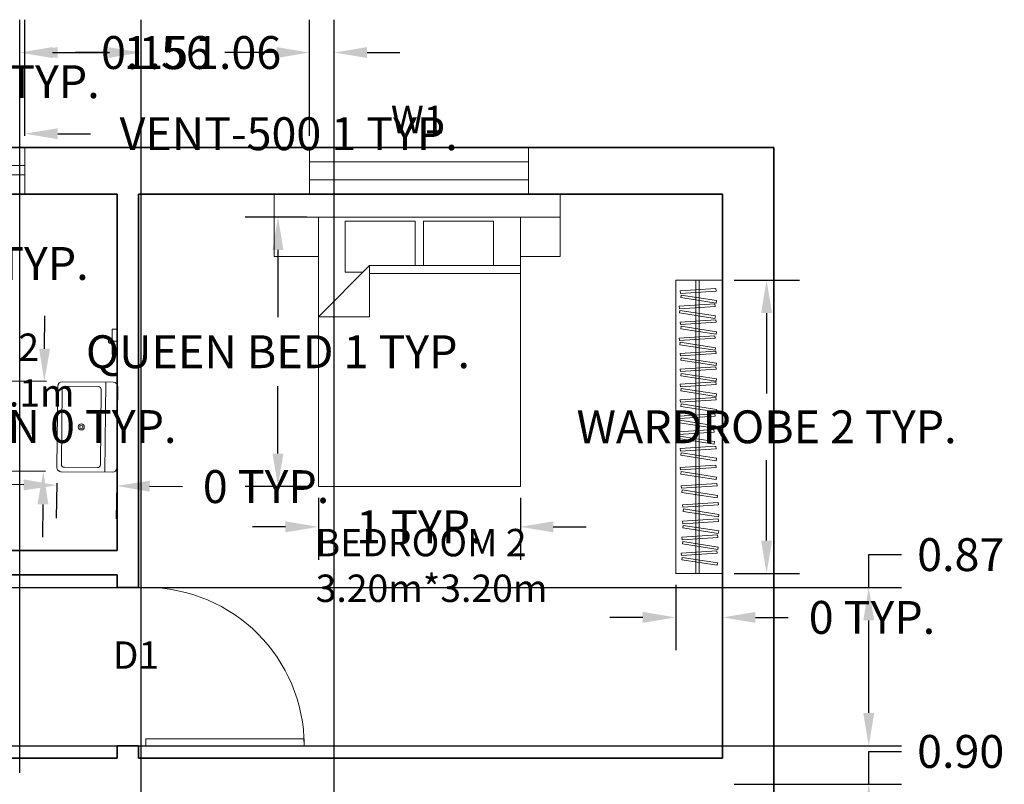
# Model space of a CAD drawing. Units: metres. Extents: x 1988.6 to 2001.1, y 2192 to 2202.5.
# Tile 6 of 6: x 1995.3 to 2000.6, y 2198.3 to 2202.5. Entities that reach past the tile are written whole.
import ezdxf

# ---------------------------------------------------------------- set-up
doc = ezdxf.new("R2010")
doc.units = ezdxf.units.M
for name, color, linetype, lineweight in [('A-ANNO-DIMS', 2, 'Continuous', 18), ('A-ANNO-TEXT', 7, 'Continuous', 18), ('A-AREA-IDEN', 7, 'Continuous', 18), ('A-DOOR', 3, 'Continuous', 18), ('A-FLOR-FIXT', 9, 'Continuous', 18), ('A-FURN', 9, 'Continuous', 15), ('A-GLAZ', 4, 'Continuous', 18), ('A-WALL', 7, 'Continuous', 35)]:
    doc.layers.add(name, color=color, linetype=linetype, lineweight=lineweight)
doc.styles.get("Standard").update_dxf_attribs({"font": 'arial.ttf'})
doc.dimstyles.get("Standard").update_dxf_attribs({"dimtxt": 0.18, "dimasz": 0.18, "dimexe": 0.18, "dimexo": 0.0625, "dimgap": 0.09, "dimtad": 0, "dimtih": 1, "dimtoh": 1, "dimdec": 4, "dimzin": 0, "dimdsep": 46, "dimtxsty": 'Standard', "dimcen": 0.09, "dimadec": 0, "dimazin": 0, "dimtfac": 1, "dimtdec": 4, "dimtofl": 0, "dimtmove": 0, "dimatfit": 3, "dimfxl": 1, "dimtolj": 1, "dimtzin": 0, "dimarcsym": 0})

# ---------------------------------------------------------------- blocks, each defined once
blk = doc.blocks.new('Bed - Queen')
for p, q in [((0, -80.00003), (0, 0)), ((0, 0), (59.99999, 0)), ((59.99999, 0), (59.99999, -80.00003)), ((7.99999, -1.2), (28.79998, -1.2)), ((7.99999, -14.4), (7.99999, -1.2)), ((28.79998, -1.2), (28.79998, -14.4)), ((31.19999, -1.2), (51.99999, -1.2)), ((31.19999, -14.4), (31.19999, -1.2)), ((51.99999, -1.2), (51.99999, -16.4)), ((0, -14.4), (44.8, -14.4)), ((59.99999, -29.6), (44.8, -14.4)), ((44.8, -14.4), (44.8, -29.6)), ((44.8, -16.8), (0, -16.8)), ((51.99999, -16.4), (46.79936, -16.4)), ((44.8, -29.6), (59.99999, -29.6)), ((59.99999, -80.00003), (0, -80.00003))]:
    blk.add_line(p, q)
blk = doc.blocks.new('Sink-single - 30 in top')
blk.add_line((-15, -3.999996), (15, -3.999996))
for points in [[(-13.5, 0), (13.5, 0)], [(-15, -18.499996), (-15, -1.5)], [(15, -1.5), (15, -18.499996)], [(-13.5, -17.499996), (-13.5, -6.499996)], [(-12.5, -5.499996), (12.5, -5.499996)], [(13.5, -6.499996), (13.5, -17.499996)], [(12.5, -18.499996), (-12.5, -18.499996)], [(13.5, -19.999996), (-13.5, -19.999996)]]:
    blk.add_lwpolyline(points)
for radius in [1, 0.5]:
    blk.add_circle((0, -11.999996), radius)
for centre, radius, start, end in [((-13.5, -1.5), 1.5, 90, 180), ((13.5, -1.5), 1.5, 0, 90), ((-12.5, -6.499996), 1, 90, 180), ((12.5, -6.499996), 1, 0, 90), ((-13.5, -18.499996), 1.5, 180, 270), ((-12.5, -17.499996), 1, 180, 270), ((12.5, -17.499996), 1, 270, 0), ((13.5, -18.499996), 1.5, 270, 0)]:
    blk.add_arc(centre, radius, start, end)
blk = doc.blocks.new('*U13')
for p, q in [((0, 0), (0, -6)), ((40, 0), (40, -6))]:
    blk.add_line(p, q)
blk.add_lwpolyline([(0, 0), (0, 40), (1.75, 40), (1.75, 0)], close=True)
blk.add_arc((0, 0), 40, 0, 90)
blk = doc.blocks.new('WIN-1200')
for p, q in [((-0.0002, 0.2568), (1.1998, 0.2568)), ((-0.0002, -0.0002), (-0.0002, 0.2568)), ((1.1998, 0.2568), (1.1998, -0.0002)), ((-0.0002, 0.1786), (1.1998, 0.1786)), ((-0.0002, 0.0793), (1.1998, 0.0793)), ((-0.0002, -0.0002), (1.1998, -0.0002))]:
    blk.add_line(p, q)
blk = doc.blocks.new('VENT-500')
for p, q in [((-0.0001, 0.2568), (-0.0001, -0.0002)), ((0.4999, 0.2568), (-0.0001, 0.2568)), ((0.4999, -0.0002), (0.4999, 0.2568)), ((0.4999, 0.1568), (-0.0001, 0.1568)), ((-0.0001, 0.1068), (0.4999, 0.1068)), ((-0.0001, -0.0002), (0.4999, -0.0002))]:
    blk.add_line(p, q)
blk = doc.blocks.new('HEADBOARD-WITH-SIDE-TABLES')
for p, q in [((-0.0002, 0.3408), (-0.0002, 0.2164)), ((1.5674, 0.2164), (1.5674, 0.3408)), ((-0.0002, 0.2164), (1.5674, 0.2164)), ((-0.0002, 0.2164), (-0.0002, 0.0002)), ((1.5674, 0.2164), (1.5674, 0.0002)), ((-0.0002, 0.0002), (0.2181, 0.0002)), ((1.5674, 0.0002), (1.3249, 0.0002))]:
    blk.add_line(p, q)
blk = doc.blocks.new('WARDROBE-HANGING')
for p, q in [((0.0001, 1.6061), (0.2571, 1.6061)), ((0.0001, 1.6061), (0.0001, 0.0002)), ((0.1103, 1.6061), (0.1103, 0.0002)), ((0.1286, 1.6061), (0.1286, 0.0002)), ((0.2571, 1.6061), (0.2571, 0.0002)), ((0.2571, 0.0002), (0.0001, 0.0002))]:
    blk.add_line(p, q)
for points in [[(0.0252, 1.5475), (0.2208, 1.5602), (0.2217, 1.5468), (0.0261, 1.5341)], [(0.0296, 1.5242), (0.2233, 1.4943), (0.2212, 1.481), (0.0275, 1.5109)], [(0.0193, 1.4638), (0.2148, 1.4765), (0.2157, 1.4631), (0.0201, 1.4504)], [(0.0236, 1.4404), (0.2173, 1.4105), (0.2153, 1.3972), (0.0216, 1.4272)], [(0.0252, 1.377), (0.2208, 1.3897), (0.2217, 1.3763), (0.0261, 1.3636)], [(0.0296, 1.3537), (0.2233, 1.3238), (0.2212, 1.3105), (0.0275, 1.3404)], [(0.0196, 1.2897), (0.2152, 1.3024), (0.2161, 1.289), (0.0205, 1.2763)], [(0.024, 1.2664), (0.2177, 1.2365), (0.2157, 1.2232), (0.022, 1.2531)], [(0.0252, 1.205), (0.2208, 1.2177), (0.2217, 1.2043), (0.0261, 1.1916)], [(0.0296, 1.1817), (0.2233, 1.1517), (0.2212, 1.1385), (0.0275, 1.1684)], [(0.0252, 1.1192), (0.2208, 1.1319), (0.2217, 1.1185), (0.0261, 1.1058)], [(0.0296, 1.0959), (0.2233, 1.066), (0.2212, 1.0527), (0.0275, 1.0827)], [(0.0252, 1.0365), (0.2208, 1.0492), (0.2217, 1.0358), (0.0261, 1.0231)], [(0.0296, 1.0132), (0.2233, 0.9833), (0.2212, 0.97), (0.0275, 0.9999)], [(0.0252, 0.9518), (0.2208, 0.9645), (0.2217, 0.9511), (0.0261, 0.9384)], [(0.0296, 0.9285), (0.2233, 0.8986), (0.2212, 0.8853), (0.0275, 0.9152)], [(0.0193, 0.8621), (0.2148, 0.8748), (0.2157, 0.8614), (0.0201, 0.8487)], [(0.0236, 0.8388), (0.2173, 0.8089), (0.2153, 0.7956), (0.0216, 0.8255)], [(0.0141, 0.7752), (0.2097, 0.7879), (0.2106, 0.7745), (0.015, 0.7618)], [(0.0185, 0.7519), (0.2122, 0.722), (0.2101, 0.7087), (0.0164, 0.7386)], [(0.0252, 0.6841), (0.2208, 0.6968), (0.2217, 0.6834), (0.0261, 0.6707)], [(0.0296, 0.6608), (0.2233, 0.6309), (0.2212, 0.6176), (0.0275, 0.6475)], [(0.0252, 0.5812), (0.2208, 0.5939), (0.2217, 0.5805), (0.0261, 0.5678)], [(0.0296, 0.5578), (0.2233, 0.5279), (0.2212, 0.5146), (0.0275, 0.5446)], [(0.0307, 0.4806), (0.2263, 0.4933), (0.2272, 0.4799), (0.0316, 0.4672)], [(0.0351, 0.4573), (0.2288, 0.4273), (0.2268, 0.4141), (0.0331, 0.444)], [(0.0379, 0.3765), (0.2335, 0.3892), (0.2344, 0.3758), (0.0388, 0.3631)], [(0.0423, 0.3532), (0.236, 0.3232), (0.2339, 0.31), (0.0403, 0.3399)], [(0.0375, 0.286), (0.2331, 0.2987), (0.234, 0.2853), (0.0384, 0.2726)], [(0.0419, 0.2627), (0.2356, 0.2327), (0.2335, 0.2195), (0.0399, 0.2494)], [(0.0342, 0.1981), (0.2298, 0.2108), (0.2307, 0.1974), (0.0351, 0.1847)], [(0.0386, 0.1748), (0.2323, 0.1448), (0.2303, 0.1316), (0.0366, 0.1615)], [(0.0307, 0.1115), (0.2263, 0.1242), (0.2272, 0.1108), (0.0316, 0.0981)], [(0.0351, 0.0882), (0.2288, 0.0583), (0.2268, 0.045), (0.0331, 0.0749)]]:
    blk.add_lwpolyline(points, close=True)
blk = doc.blocks.new('BATH-WALL-FITTING')
for p, q in [((-0.0001, 0.0002), (-0.0001, 0.138)), ((-0.0001, 0.138), (0.028, 0.138)), ((0.028, 0.1375), (0.028, 0.0002)), ((-0.0001, 0.0715), (0.028, 0.0715)), ((0.028, 0.0002), (-0.0001, 0.0002))]:
    blk.add_line(p, q)
blk.add_circle((0.0382, 0.0715), 0.0103)
blk = doc.blocks.new('*D24')
at = {"layer": 'A-ANNO-DIMS', "color": 0, "lineweight": -2, "transparency": 16777216}
for p, q in [((1996.824, 2201.3724), (1996.4852, 2201.3724)), ((1996.6652, 2201.1924), (1996.6652, 2200.8231)), ((1996.6652, 2200.0767), (1996.6652, 2200.4459)), ((1996.824, 2199.8967), (1996.4852, 2199.8967))]:
    blk.add_line(p, q, dxfattribs=at)
at = {"layer": 'A-ANNO-DIMS', "color": 0, "transparency": 16777216}
for points in [[(1996.6352, 2201.1924), (1996.6952, 2201.1924), (1996.6652, 2201.3724)], [(1996.6352, 2200.0767), (1996.6952, 2200.0767), (1996.6652, 2199.8967)]]:
    blk.add_solid(points, dxfattribs=at)
at = {"layer": 'Defpoints', "color": 0, "transparency": 16777216}
for p in [(1996.6652, 2201.3724), (1996.8865, 2201.3724), (1996.8865, 2199.8967)]:
    blk.add_point(p, dxfattribs=at)
at = {"layer": 'A-ANNO-DIMS', "color": 0, "transparency": 16777216, "insert": (1996.6652, 2200.6345), "char_height": 0.18, "attachment_point": 5}
blk.add_mtext('\\A1;QUEEN BED 1 TYP.', dxfattribs=at)
blk = doc.blocks.new('*D25')
at = {"layer": 'A-ANNO-DIMS', "color": 0, "lineweight": -2, "transparency": 16777216}
for p, q in [((1996.8865, 2199.8342), (1996.8865, 2199.4954)), ((1997.9932, 2199.8342), (1997.9932, 2199.4954)), ((1996.7065, 2199.6754), (1996.5265, 2199.6754)), ((1998.1732, 2199.6754), (1998.3532, 2199.6754))]:
    blk.add_line(p, q, dxfattribs=at)
at = {"layer": 'A-ANNO-DIMS', "color": 0, "transparency": 16777216}
for points in [[(1996.7065, 2199.7054), (1996.7065, 2199.6454), (1996.8865, 2199.6754)], [(1998.1732, 2199.7054), (1998.1732, 2199.6454), (1997.9932, 2199.6754)]]:
    blk.add_solid(points, dxfattribs=at)
at = {"layer": 'Defpoints', "color": 0, "transparency": 16777216}
for p in [(1996.8865, 2199.8967), (1997.9932, 2199.8967), (1996.8865, 2199.6754)]:
    blk.add_point(p, dxfattribs=at)
at = {"layer": 'A-ANNO-DIMS', "color": 0, "transparency": 16777216, "insert": (1997.4399, 2199.6754), "char_height": 0.18, "attachment_point": 5}
blk.add_mtext('\\A1;1 TYP.', dxfattribs=at)
blk = doc.blocks.new('*D28')
at = {"layer": 'A-ANNO-DIMS', "color": 0, "lineweight": -2, "transparency": 16777216}
for p, q in [((1995.3871, 2200.6513), (1995.3891, 2200.8313)), ((1995.3967, 2200.4712), (1995.2052, 2200.4733)), ((1995.3914, 2199.9779), (1995.1999, 2199.98)), ((1995.3779, 2199.7981), (1995.376, 2199.6181))]:
    blk.add_line(p, q, dxfattribs=at)
at = {"layer": 'A-ANNO-DIMS', "color": 0, "transparency": 16777216}
for points in [[(1995.3571, 2200.6517), (1995.4171, 2200.651), (1995.3852, 2200.4714)], [(1995.3479, 2199.7984), (1995.4079, 2199.7978), (1995.3799, 2199.9781)]]:
    blk.add_solid(points, dxfattribs=at)
at = {"layer": 'Defpoints', "color": 0, "transparency": 16777216}
for p in [(1995.4592, 2200.4706), (1995.3799, 2199.9781), (1995.4538, 2199.9773)]:
    blk.add_point(p, dxfattribs=at)
at = {"layer": 'A-ANNO-DIMS', "color": 0, "transparency": 16777216, "insert": (1995.3825, 2200.2247), "char_height": 0.18, "attachment_point": 5}
blk.add_mtext('\\A1;BASIN 0 TYP.', dxfattribs=at)
blk = doc.blocks.new('*D29')
at = {"layer": 'A-ANNO-DIMS', "color": 0, "lineweight": -2, "transparency": 16777216}
for p, q in [((1995.2731, 2199.9052), (1995.0931, 2199.9072)), ((1995.4532, 2199.9148), (1995.4511, 2199.7233)), ((1995.782, 2199.9112), (1995.78, 2199.7197)), ((1995.9619, 2199.8978), (1996.1419, 2199.8958))]:
    blk.add_line(p, q, dxfattribs=at)
at = {"layer": 'A-ANNO-DIMS', "color": 0, "transparency": 16777216}
for points in [[(1995.2734, 2199.9352), (1995.2727, 2199.8752), (1995.453, 2199.9033)], [(1995.9622, 2199.9278), (1995.9616, 2199.8678), (1995.7819, 2199.8997)]]:
    blk.add_solid(points, dxfattribs=at)
at = {"layer": 'Defpoints', "color": 0, "transparency": 16777216}
for p in [(1995.4538, 2199.9773), (1995.7827, 2199.9737), (1995.7819, 2199.8997)]:
    blk.add_point(p, dxfattribs=at)
at = {"layer": 'A-ANNO-DIMS', "color": 0, "transparency": 16777216, "insert": (1996.6, 2199.8958), "char_height": 0.18, "attachment_point": 5}
blk.add_mtext('\\A1;0 TYP.', dxfattribs=at)
blk = doc.blocks.new('*D34')
at = {"layer": 'A-ANNO-DIMS', "color": 0, "lineweight": -2, "transparency": 16777216}
for p, q in [((1994.7792, 2201.8163), (1994.7792, 2202.0088)), ((1995.2792, 2201.8163), (1995.2792, 2202.0088)), ((1994.5992, 2201.8288), (1994.4192, 2201.8288)), ((1995.4592, 2201.8288), (1995.6392, 2201.8288))]:
    blk.add_line(p, q, dxfattribs=at)
at = {"layer": 'A-ANNO-DIMS', "color": 0, "transparency": 16777216}
for points in [[(1994.5992, 2201.8588), (1994.5992, 2201.7988), (1994.7792, 2201.8288)], [(1995.4592, 2201.8588), (1995.4592, 2201.7988), (1995.2792, 2201.8288)]]:
    blk.add_solid(points, dxfattribs=at)
at = {"layer": 'Defpoints', "color": 0, "transparency": 16777216}
for p in [(1995.2792, 2201.8288), (1994.7792, 2201.7538), (1995.2792, 2201.7538)]:
    blk.add_point(p, dxfattribs=at)
at = {"layer": 'A-ANNO-DIMS', "color": 0, "transparency": 16777216, "insert": (1996.724, 2201.8288), "char_height": 0.18, "attachment_point": 5}
blk.add_mtext('\\A1;VENT-500 1 TYP.', dxfattribs=at)
blk = doc.blocks.new('*D35')
at = {"layer": 'A-ANNO-DIMS', "color": 0, "lineweight": -2, "transparency": 16777216}
for p, q in [((1994.7042, 2201.9338), (1994.7042, 2202.1138)), ((1994.7042, 2202.1138), (1994.8842, 2202.1138)), ((1994.7167, 2201.7538), (1994.5242, 2201.7538)), ((1994.7167, 2201.4968), (1994.5242, 2201.4968)), ((1994.7042, 2201.3168), (1994.7042, 2201.1368))]:
    blk.add_line(p, q, dxfattribs=at)
at = {"layer": 'A-ANNO-DIMS', "color": 0, "transparency": 16777216}
for points in [[(1994.6742, 2201.9338), (1994.7342, 2201.9338), (1994.7042, 2201.7538)], [(1994.6742, 2201.3168), (1994.7342, 2201.3168), (1994.7042, 2201.4968)]]:
    blk.add_solid(points, dxfattribs=at)
at = {"layer": 'Defpoints', "color": 0, "transparency": 16777216}
for p in [(1994.7042, 2201.7538), (1994.7792, 2201.7538), (1994.7792, 2201.4968)]:
    blk.add_point(p, dxfattribs=at)
at = {"layer": 'A-ANNO-DIMS', "color": 0, "transparency": 16777216, "insert": (1995.3424, 2202.1138), "char_height": 0.18, "attachment_point": 5}
blk.add_mtext('\\A1;0 TYP.', dxfattribs=at)
blk = doc.blocks.new('*D38')
at = {"layer": 'A-ANNO-DIMS', "color": 0, "lineweight": -2, "transparency": 16777216}
for p, q in [((1999.1632, 2201.0261), (1999.5216, 2201.0261)), ((1999.3416, 2200.8461), (1999.3416, 2200.4063)), ((1999.3416, 2199.6002), (1999.3416, 2200.04)), ((1999.1632, 2199.4202), (1999.5216, 2199.4202))]:
    blk.add_line(p, q, dxfattribs=at)
at = {"layer": 'A-ANNO-DIMS', "color": 0, "transparency": 16777216}
for points in [[(1999.3116, 2200.8461), (1999.3716, 2200.8461), (1999.3416, 2201.0261)], [(1999.3116, 2199.6002), (1999.3716, 2199.6002), (1999.3416, 2199.4202)]]:
    blk.add_solid(points, dxfattribs=at)
at = {"layer": 'Defpoints', "color": 0, "transparency": 16777216}
for p in [(1999.1007, 2201.0261), (1999.3416, 2201.0261), (1999.1007, 2199.4202)]:
    blk.add_point(p, dxfattribs=at)
at = {"layer": 'A-ANNO-DIMS', "color": 0, "transparency": 16777216, "insert": (1999.3416, 2200.2232), "char_height": 0.18, "attachment_point": 5}
blk.add_mtext('\\A1;WARDROBE 2 TYP.', dxfattribs=at)
blk = doc.blocks.new('*D39')
at = {"layer": 'A-ANNO-DIMS', "color": 0, "lineweight": -2, "transparency": 16777216}
for p, q in [((1998.8437, 2199.3577), (1998.8437, 2198.9993)), ((1999.1007, 2199.3577), (1999.1007, 2198.9993)), ((1998.6637, 2199.1793), (1998.4837, 2199.1793)), ((1999.2807, 2199.1793), (1999.4607, 2199.1793))]:
    blk.add_line(p, q, dxfattribs=at)
at = {"layer": 'A-ANNO-DIMS', "color": 0, "transparency": 16777216}
for points in [[(1998.6637, 2199.2093), (1998.6637, 2199.1493), (1998.8437, 2199.1793)], [(1999.2807, 2199.2093), (1999.2807, 2199.1493), (1999.1007, 2199.1793)]]:
    blk.add_solid(points, dxfattribs=at)
at = {"layer": 'Defpoints', "color": 0, "transparency": 16777216}
for p in [(1998.8437, 2199.4202), (1999.1007, 2199.4202), (1999.1007, 2199.1793)]:
    blk.add_point(p, dxfattribs=at)
at = {"layer": 'A-ANNO-DIMS', "color": 0, "transparency": 16777216, "insert": (1999.9188, 2199.1793), "char_height": 0.18, "attachment_point": 5}
blk.add_mtext('\\A1;0 TYP.', dxfattribs=at)
blk = doc.blocks.new('*D42')
at = {"layer": 'A-ANNO-DIMS', "color": 0, "lineweight": -2, "transparency": 16777216}
for p, q in [((1992.9081, 2200.938), (1992.9081, 2201.118)), ((1992.9081, 2201.118), (1993.0881, 2201.118)), ((1992.95, 2200.758), (1993.0881, 2200.758)), ((1992.95, 2200.6202), (1993.0881, 2200.6202)), ((1992.9081, 2200.4402), (1992.9081, 2200.2602))]:
    blk.add_line(p, q, dxfattribs=at)
at = {"layer": 'A-ANNO-DIMS', "color": 0, "transparency": 16777216}
for points in [[(1992.8781, 2200.938), (1992.9381, 2200.938), (1992.9081, 2200.758)], [(1992.8781, 2200.4402), (1992.9381, 2200.4402), (1992.9081, 2200.6202)]]:
    blk.add_solid(points, dxfattribs=at)
at = {"layer": 'Defpoints', "color": 0, "transparency": 16777216}
for p in [(1992.8875, 2200.758), (1992.9081, 2200.758), (1992.8875, 2200.6202)]:
    blk.add_point(p, dxfattribs=at)
at = {"layer": 'A-ANNO-DIMS', "color": 0, "transparency": 16777216, "insert": (1994.4511, 2201.118), "char_height": 0.18, "attachment_point": 5}
blk.add_mtext('\\A1;WALL FITTING 0 TYP.', dxfattribs=at)
blk = doc.blocks.new('*D57')
at = {"layer": 'A-ANNO-DIMS', "color": 0, "lineweight": -2, "transparency": 16777216}
for p, q in [((1995.2792, 2201.8163), (1995.2792, 2202.4533)), ((1996.8377, 2201.8163), (1996.8377, 2202.4533)), ((1995.4592, 2202.2733), (1995.7433, 2202.2733)), ((1996.6577, 2202.2733), (1996.3737, 2202.2733))]:
    blk.add_line(p, q, dxfattribs=at)
at = {"layer": 'A-ANNO-DIMS', "color": 0, "transparency": 16777216}
for points in [[(1995.4592, 2202.3033), (1995.4592, 2202.2433), (1995.2792, 2202.2733)], [(1996.6577, 2202.3033), (1996.6577, 2202.2433), (1996.8377, 2202.2733)]]:
    blk.add_solid(points, dxfattribs=at)
at = {"layer": 'Defpoints', "color": 0, "transparency": 16777216}
for p in [(1996.8377, 2202.2733), (1995.2792, 2201.7538), (1996.8377, 2201.7538)]:
    blk.add_point(p, dxfattribs=at)
at = {"layer": 'A-ANNO-DIMS', "color": 0, "transparency": 16777216, "insert": (1996.0585, 2202.2733), "char_height": 0.18, "attachment_point": 5}
blk.add_mtext('\\A1;1.56', dxfattribs=at)
blk = doc.blocks.new('*D71')
at = {"layer": 'A-ANNO-DIMS', "color": 0, "lineweight": -2, "transparency": 16777216}
for p, q in [((1999.9013, 2198.2651), (1999.9013, 2198.4451)), ((1999.9013, 2198.4451), (2000.0813, 2198.4451)), ((1999.1632, 2198.2651), (2000.0813, 2198.2651)), ((1999.9013, 2197.5493), (1999.9013, 2198.0851)), ((1999.4443, 2197.3693), (2000.0813, 2197.3693))]:
    blk.add_line(p, q, dxfattribs=at)
at = {"layer": 'A-ANNO-DIMS', "color": 0, "transparency": 16777216}
for points in [[(1999.8713, 2198.0851), (1999.9313, 2198.0851), (1999.9013, 2198.2651)], [(1999.8713, 2197.5493), (1999.9313, 2197.5493), (1999.9013, 2197.3693)]]:
    blk.add_solid(points, dxfattribs=at)
at = {"layer": 'Defpoints', "color": 0, "transparency": 16777216}
for p in [(1999.1007, 2198.2651), (1999.9013, 2198.2651), (1999.3818, 2197.3693)]:
    blk.add_point(p, dxfattribs=at)
at = {"layer": 'A-ANNO-DIMS', "color": 0, "transparency": 16777216, "insert": (2000.4048, 2198.4451), "char_height": 0.18, "attachment_point": 5}
blk.add_mtext('\\A1;0.90', dxfattribs=at)
blk = doc.blocks.new('*D72')
at = {"layer": 'A-ANNO-DIMS', "color": 0, "lineweight": -2, "transparency": 16777216}
for p, q in [((1999.9013, 2199.3431), (1999.9013, 2199.5231)), ((1999.9013, 2199.5231), (2000.0813, 2199.5231)), ((1992.7483, 2199.3431), (2000.0813, 2199.3431)), ((1999.9013, 2198.656), (1999.9013, 2199.1631)), ((1992.7483, 2198.476), (2000.0813, 2198.476))]:
    blk.add_line(p, q, dxfattribs=at)
at = {"layer": 'A-ANNO-DIMS', "color": 0, "transparency": 16777216}
for points in [[(1999.8713, 2199.1631), (1999.9313, 2199.1631), (1999.9013, 2199.3431)], [(1999.8713, 2198.656), (1999.9313, 2198.656), (1999.9013, 2198.476)]]:
    blk.add_solid(points, dxfattribs=at)
at = {"layer": 'Defpoints', "color": 0, "transparency": 16777216}
for p in [(1992.6858, 2199.3431), (1999.9013, 2199.3431), (1992.6858, 2198.476)]:
    blk.add_point(p, dxfattribs=at)
at = {"layer": 'A-ANNO-DIMS', "color": 0, "transparency": 16777216, "insert": (2000.4051, 2199.5231), "char_height": 0.18, "attachment_point": 5}
blk.add_mtext('\\A1;0.87', dxfattribs=at)
blk = doc.blocks.new('*D74')
at = {"layer": 'A-ANNO-DIMS', "color": 0, "lineweight": -2, "transparency": 16777216}
for p, q in [((1995.9155, 2195.9076), (1995.9155, 2202.4533)), ((1996.9733, 2195.9076), (1996.9733, 2202.4533)), ((1995.7355, 2202.2733), (1995.5555, 2202.2733)), ((1997.1533, 2202.2733), (1997.3333, 2202.2733))]:
    blk.add_line(p, q, dxfattribs=at)
at = {"layer": 'A-ANNO-DIMS', "color": 0, "transparency": 16777216}
for points in [[(1995.7355, 2202.3033), (1995.7355, 2202.2433), (1995.9155, 2202.2733)], [(1997.1533, 2202.3033), (1997.1533, 2202.2433), (1996.9733, 2202.2733)]]:
    blk.add_solid(points, dxfattribs=at)
at = {"layer": 'Defpoints', "color": 0, "transparency": 16777216}
for p in [(1996.9733, 2202.2733), (1995.9155, 2195.8451), (1996.9733, 2195.8451)]:
    blk.add_point(p, dxfattribs=at)
at = {"layer": 'A-ANNO-DIMS', "color": 0, "transparency": 16777216, "insert": (1996.4444, 2202.2733), "char_height": 0.18, "attachment_point": 5}
blk.add_mtext('\\A1;1.06', dxfattribs=at)
blk = doc.blocks.new('*D75')
at = {"layer": 'A-ANNO-DIMS', "color": 0, "lineweight": -2, "transparency": 16777216}
for p, q in [((1995.1007, 2198.4713), (1995.1007, 2202.4533)), ((1995.2507, 2198.3276), (1995.2507, 2202.4533)), ((1994.9207, 2202.2733), (1994.7407, 2202.2733)), ((1995.4307, 2202.2733), (1995.6107, 2202.2733))]:
    blk.add_line(p, q, dxfattribs=at)
at = {"layer": 'A-ANNO-DIMS', "color": 0, "transparency": 16777216}
for points in [[(1994.9207, 2202.3033), (1994.9207, 2202.2433), (1995.1007, 2202.2733)], [(1995.4307, 2202.3033), (1995.4307, 2202.2433), (1995.2507, 2202.2733)]]:
    blk.add_solid(points, dxfattribs=at)
at = {"layer": 'Defpoints', "color": 0, "transparency": 16777216}
for p in [(1995.2507, 2202.2733), (1995.1007, 2198.4088), (1995.2507, 2198.2651)]:
    blk.add_point(p, dxfattribs=at)
at = {"layer": 'A-ANNO-DIMS', "color": 0, "transparency": 16777216, "insert": (1995.9351, 2202.2733), "char_height": 0.18, "attachment_point": 5}
blk.add_mtext('\\A1;0.15', dxfattribs=at)

msp = doc.modelspace()

# ---------------------------------------------------------------- linework, layer by layer
at = {"layer": 'A-WALL'}
for p, q in [((1999.3818, 2201.7538), (1989.3818, 2201.7538)), ((1999.3818, 2192.7038), (1999.3818, 2201.7538)), ((1995.7849, 2201.4968), (1994.36, 2201.4968)), ((1995.7849, 2201.4968), (1995.7849, 2199.545)), ((1999.1007, 2201.4968), (1995.902, 2201.4968)), ((1995.902, 2201.4968), (1995.902, 2199.3431)), ((1999.1007, 2198.4088), (1999.1007, 2201.4968)), ((1995.7849, 2199.545), (1995.0418, 2199.545)), ((1995.7849, 2199.412), (1995.0418, 2199.412)), ((1995.7849, 2199.412), (1995.7849, 2199.3431)), ((1995.902, 2199.3431), (1995.7849, 2199.3431)), ((1995.7847, 2198.476), (1995.7849, 2198.4088)), ((1995.902, 2198.476), (1995.7847, 2198.476)), ((1995.902, 2198.476), (1995.902, 2198.4088)), ((1995.7849, 2198.4088), (1995.1007, 2198.4088)), ((1999.1007, 2198.4088), (1995.902, 2198.4088))]:
    msp.add_line(p, q, dxfattribs=at)

# ---------------------------------------------------------------- block references
at = {"layer": 'A-DOOR', "xscale": -0.021677520635372, "yscale": 0.021677520635372, "zscale": 0.021677520635372, "rotation": 270}
msp.add_blockref('*U13', (1995.9419, 2198.476), dxfattribs=at)
at = {"layer": 'A-FLOR-FIXT', "extrusion": (0, 0, -1), "zscale": -1}
msp.add_blockref('BATH-WALL-FITTING', (-1995.7848, 2200.62), dxfattribs=at)
at = {"layer": 'A-FLOR-FIXT', "xscale": 0.0164438288540887, "yscale": 0.0164438288540887, "zscale": 0.0164438288540887, "rotation": 269.3807925307475}
msp.add_blockref('Sink-single - 30 in top', (1995.7854, 2200.2204), dxfattribs=at)
at = {"layer": 'A-FURN', "extrusion": (0, 0, -1), "zscale": -1}
msp.add_blockref('HEADBOARD-WITH-SIDE-TABLES', (-1998.2114, 2201.156), dxfattribs=at)
at = {"layer": 'A-FURN', "xscale": -0.0184456424226754, "yscale": 0.0184456424226754, "zscale": 0.0184456424226754}
msp.add_blockref('Bed - Queen', (1997.9932, 2201.3724), dxfattribs=at)
at = {"layer": 'A-FURN'}
msp.add_blockref('WARDROBE-HANGING', (1998.8436, 2199.42), dxfattribs=at)
at = {"layer": 'A-GLAZ'}
for name, p in [('VENT-500', (1994.7794, 2201.497)), ('WIN-1200', (1996.838, 2201.497))]:
    msp.add_blockref(name, p, dxfattribs=at)

# ---------------------------------------------------------------- texts
at = {"layer": 'A-ANNO-TEXT', "char_height": 0.15, "attachment_point": 1}
for s, insert in [('W1', (1997.2841, 2201.9816)), ('D1', (1995.7605, 2199.048))]:
    msp.add_mtext_dynamic_manual_height_columns(s, width=0.386628, gutter_width=12.5, heights=[0], dxfattribs=dict(at, insert=insert))
at = {"layer": 'A-AREA-IDEN', "char_height": 0.15, "attachment_point": 1}
for s, width, insert in [('TOILET 2\\P1.5m*2.1m', 1.378048, (1994.5087, 2200.7343)), ('BEDROOM 2\\P3.20m*3.20m', 1.796061, (1996.8717, 2199.6639))]:
    msp.add_mtext_dynamic_manual_height_columns(s, width=width, gutter_width=12.5, heights=[0], dxfattribs=dict(at, insert=insert))

# ---------------------------------------------------------------- dimensions: what is measured, and where the dimension line sits
at = {"layer": 'A-ANNO-DIMS'}
for base, p1, p2, picture, middle in [((1995.2507, 2202.2733), (1995.1007, 2198.4088), (1995.2507, 2198.2651), '*D75', (1995.9351, 2202.2733)), ((1996.8377, 2202.2733), (1995.2792, 2201.7538), (1996.8377, 2201.7538), '*D57', (1996.0585, 2202.2733)), ((1996.9733, 2202.2733), (1995.9155, 2195.8451), (1996.9733, 2195.8451), '*D74', (1996.4444, 2202.2733))]:
    dim = msp.add_linear_dim(base=base, p1=p1, p2=p2, dimstyle='Standard', override={"dimdec": 2, "dimlfac": 1, "dimrnd": 0, "dimzin": 0, "dimdsep": 46, "dimlunit": 2}, dxfattribs=at)
    dim.commit()
    dim.dimension.update_dxf_attribs({"geometry": picture, "text_midpoint": middle})
for base, p1, p2, angle, text, picture, middle in [((1994.7042, 2201.7538), (1994.7792, 2201.4968), (1994.7792, 2201.7538), 90, '<> TYP.', '*D35', (1995.3424, 2202.1138)), ((1992.9081, 2200.758), (1992.8875, 2200.6202), (1992.8875, 2200.758), 90, 'WALL FITTING <> TYP.', '*D42', (1994.4511, 2201.118)), ((1996.6652, 2201.3724), (1996.8865, 2199.8967), (1996.8865, 2201.3724), 90, 'QUEEN BED <> TYP.', '*D24', (1996.6652, 2200.6345)), ((1999.3416, 2201.0261), (1999.1007, 2199.4202), (1999.1007, 2201.0261), 90, 'WARDROBE <> TYP.', '*D38', (1999.3416, 2200.2232)), ((1995.3799, 2199.9781), (1995.4592, 2200.4706), (1995.4538, 2199.9773), 269.3808, 'BASIN <> TYP.', '*D28', (1995.3825, 2200.2247)), ((1995.7819, 2199.8997), (1995.4538, 2199.9773), (1995.7827, 2199.9737), 359.3808, '<> TYP.', '*D29', (1996.6, 2199.8958)), ((1996.8865, 2199.6754), (1997.9932, 2199.8967), (1996.8865, 2199.8967), 180, '<> TYP.', '*D25', (1997.4399, 2199.6754))]:
    dim = msp.add_linear_dim(base=base, p1=p1, p2=p2, angle=angle, text=text, dimstyle='Standard', override={"dimdec": 0, "dimlfac": 1, "dimrnd": 0, "dimzin": 0, "dimdsep": 46, "dimlunit": 2}, dxfattribs=at)
    dim.commit()
    dim.dimension.update_dxf_attribs({"geometry": picture, "text_midpoint": middle})
for base, p1, p2, text, picture, middle in [((1995.279249203, 2201.8288284845), (1994.779249203, 2201.7538284845), (1995.279249203, 2201.7538284845), 'VENT-500 <> TYP.', '*D34', (1996.7239763517, 2201.8288284845)), ((1999.1007, 2199.1793), (1998.8437, 2199.4202), (1999.1007, 2199.4202), '<> TYP.', '*D39', (1999.9188, 2199.1793))]:
    dim = msp.add_linear_dim(base=base, p1=p1, p2=p2, text=text, dimstyle='Standard', override={"dimdec": 0, "dimlfac": 1, "dimrnd": 0, "dimzin": 0, "dimdsep": 46, "dimlunit": 2}, dxfattribs=at)
    dim.commit()
    dim.dimension.update_dxf_attribs({"geometry": picture, "text_midpoint": middle})
for base, p1, p2, picture, middle in [((1999.9013, 2199.3431), (1992.6858, 2198.476), (1992.6858, 2199.3431), '*D72', (2000.4051, 2199.5231)), ((1999.9013, 2198.2651), (1999.3818, 2197.3693), (1999.1007, 2198.2651), '*D71', (2000.4048, 2198.4451))]:
    dim = msp.add_linear_dim(base=base, p1=p1, p2=p2, angle=90, dimstyle='Standard', override={"dimdec": 2, "dimlfac": 1, "dimrnd": 0, "dimzin": 0, "dimdsep": 46, "dimlunit": 2}, dxfattribs=at)
    dim.commit()
    dim.dimension.update_dxf_attribs({"geometry": picture, "text_midpoint": middle})

doc.saveas('drawing.dxf')
